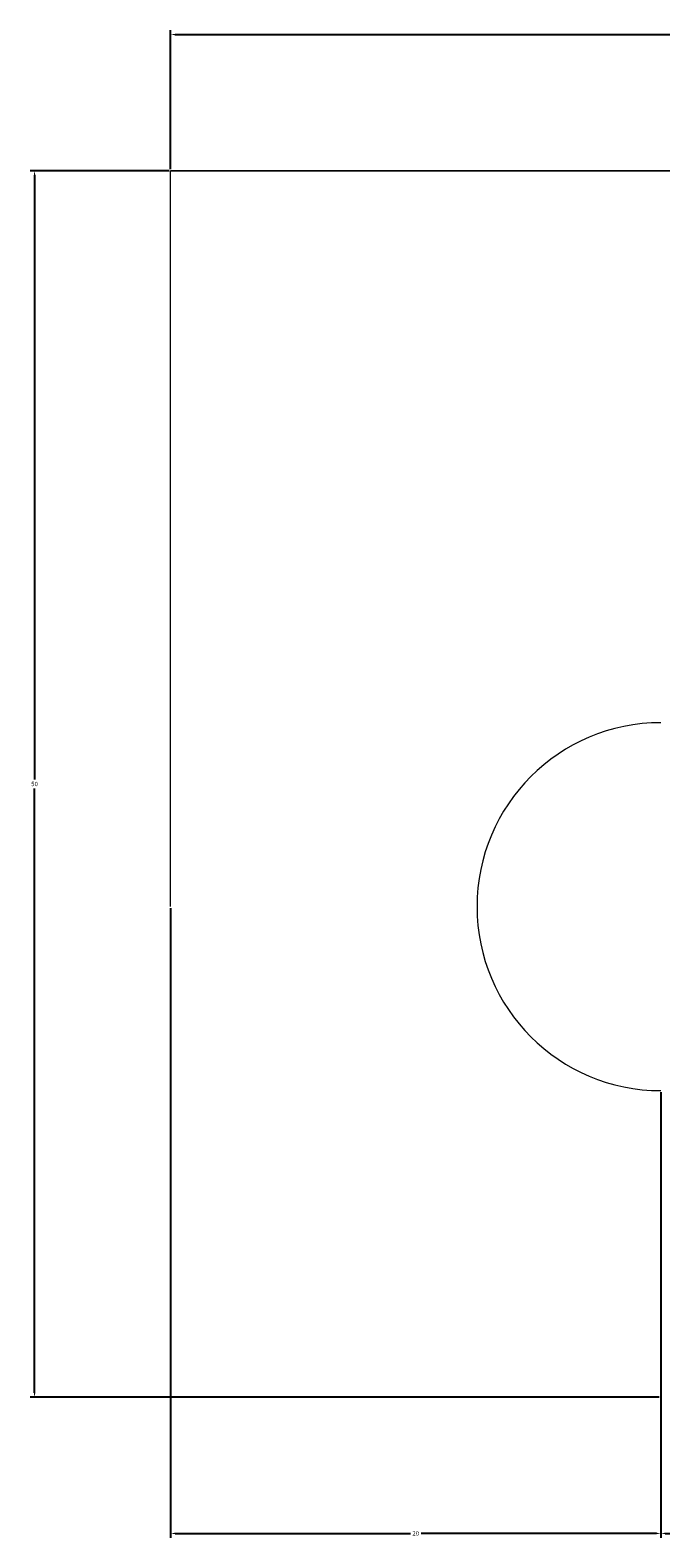
# Model space of a CAD drawing. Units: millimetres. Extents: x 88 to 204, y -56 to 6.
# Tile 1 of 3: x 88 to 114, y -56 to 6. Entities that reach past the tile are written whole.
import ezdxf

# ---------------------------------------------------------------- set-up
doc = ezdxf.new("R2010")
doc.units = ezdxf.units.MM
doc.layers.add('M-CONS', color=8, linetype='Continuous', lineweight=13)
doc.layers.add('M-DIMS', color=2, linetype='Continuous', lineweight=18)
doc.styles.get("Standard").update_dxf_attribs({"font": 'arial.ttf'})
doc.dimstyles.get("Standard").update_dxf_attribs({"dimtxt": 0.18, "dimasz": 0.18, "dimexe": 0.18, "dimexo": 0.0625, "dimgap": 0.09, "dimtad": 0, "dimtih": 1, "dimtoh": 1, "dimdec": 4, "dimzin": 0, "dimdsep": 46, "dimtxsty": 'Standard', "dimcen": 0.09, "dimadec": 0, "dimazin": 0, "dimtfac": 1, "dimtdec": 4, "dimtofl": 0, "dimtmove": 0, "dimatfit": 3, "dimfxl": 1, "dimtolj": 1, "dimtzin": 0, "dimarcsym": 0})

# ---------------------------------------------------------------- blocks, each defined once
blk = doc.blocks.new('*D1')
at = {"layer": 'Defpoints', "color": 0, "transparency": 16777216}
for p in [(198.717, 5.55), (93.717, 0), (198.717, 0)]:
    blk.add_point(p, dxfattribs=at)
at = {"layer": 'M-DIMS', "color": 0, "lineweight": -2, "transparency": 16777216}
for p, q in [((93.717, 0.062), (93.717, 5.73)), ((93.897, 5.55), (145.936, 5.55)), ((198.537, 5.55), (146.498, 5.55)), ((198.717, 0.062), (198.717, 5.73))]:
    blk.add_line(p, q, dxfattribs=at)
at = {"layer": 'M-DIMS', "color": 0, "transparency": 16777216}
for points in [[(93.897, 5.58), (93.897, 5.52), (93.717, 5.55)], [(198.537, 5.58), (198.537, 5.52), (198.717, 5.55)]]:
    blk.add_solid(points, dxfattribs=at)
at = {"layer": 'M-DIMS', "color": 0, "transparency": 16777216, "insert": (146.217, 5.55), "char_height": 0.18, "attachment_point": 5}
blk.add_mtext('\\A1;105', dxfattribs=at)
blk = doc.blocks.new('*D2')
at = {"layer": 'Defpoints', "color": 0, "transparency": 16777216}
for p in [(93.717, 0), (88.167, -50), (113.717, -50)]:
    blk.add_point(p, dxfattribs=at)
at = {"layer": 'M-DIMS', "color": 0, "lineweight": -2, "transparency": 16777216}
for p, q in [((93.654, 0), (87.987, 0)), ((88.167, -0.18), (88.167, -24.818)), ((88.167, -49.82), (88.167, -25.182)), ((113.654, -50), (87.987, -50))]:
    blk.add_line(p, q, dxfattribs=at)
at = {"layer": 'M-DIMS', "color": 0, "transparency": 16777216}
for points in [[(88.137, -0.18), (88.197, -0.18), (88.167, 0)], [(88.137, -49.82), (88.197, -49.82), (88.167, -50)]]:
    blk.add_solid(points, dxfattribs=at)
at = {"layer": 'M-DIMS', "color": 0, "transparency": 16777216, "insert": (88.167, -25), "char_height": 0.18, "attachment_point": 5}
blk.add_mtext('\\A1;50', dxfattribs=at)
blk = doc.blocks.new('*D3')
at = {"layer": 'Defpoints', "color": 0, "transparency": 16777216}
for p in [(93.717, -30), (113.717, -50), (113.717, -55.55)]:
    blk.add_point(p, dxfattribs=at)
at = {"layer": 'M-DIMS', "color": 0, "lineweight": -2, "transparency": 16777216}
for p, q in [((93.717, -30.062), (93.717, -55.73)), ((113.717, -50.062), (113.717, -55.73)), ((93.897, -55.55), (103.497, -55.55)), ((113.537, -55.55), (103.937, -55.55))]:
    blk.add_line(p, q, dxfattribs=at)
at = {"layer": 'M-DIMS', "color": 0, "transparency": 16777216}
for points in [[(93.897, -55.52), (93.897, -55.58), (93.717, -55.55)], [(113.537, -55.52), (113.537, -55.58), (113.717, -55.55)]]:
    blk.add_solid(points, dxfattribs=at)
at = {"layer": 'M-DIMS', "color": 0, "transparency": 16777216, "insert": (103.717, -55.55), "char_height": 0.18, "attachment_point": 5}
blk.add_mtext('\\A1;20', dxfattribs=at)
blk = doc.blocks.new('*D4')
at = {"layer": 'Defpoints', "color": 0, "transparency": 16777216}
for p in [(113.717, -37.5), (143.717, -37.5), (143.717, -55.55)]:
    blk.add_point(p, dxfattribs=at)
at = {"layer": 'M-DIMS', "color": 0, "lineweight": -2, "transparency": 16777216}
for p, q in [((113.717, -37.562), (113.717, -55.73)), ((143.717, -37.562), (143.717, -55.73)), ((113.897, -55.55), (128.498, -55.55)), ((143.537, -55.55), (128.935, -55.55))]:
    blk.add_line(p, q, dxfattribs=at)
at = {"layer": 'M-DIMS', "color": 0, "transparency": 16777216}
for points in [[(113.897, -55.52), (113.897, -55.58), (113.717, -55.55)], [(143.537, -55.52), (143.537, -55.58), (143.717, -55.55)]]:
    blk.add_solid(points, dxfattribs=at)
at = {"layer": 'M-DIMS', "color": 0, "transparency": 16777216, "insert": (128.717, -55.55), "char_height": 0.18, "attachment_point": 5}
blk.add_mtext('\\A1;30', dxfattribs=at)

msp = doc.modelspace()

# ---------------------------------------------------------------- linework, layer by layer
at = {"layer": 'M-CONS', "extrusion": (0, -1, 0)}
for p, q in [((163.717, 0, 52.588), (93.717, 0, 52.588)), ((93.717, 0, 72.588), (163.717, 0, 72.588)), ((93.717, 0, 72.588), (93.717, 0, 112.588))]:
    msp.add_line(p, q, dxfattribs=at)
at = {"layer": 'M-CONS'}
for p, q in [((93.717, 0, 52.588), (93.717, 0, 62.588)), ((93.717, 0, 62.588), (163.717, 0, 62.588)), ((93.717, -30, 62.588), (93.717, 0, 62.588))]:
    msp.add_line(p, q, dxfattribs=at)
msp.add_arc((113.717, -30, 62.588), 7.5, 90, 270, dxfattribs=at)

# ---------------------------------------------------------------- dimensions: what is measured, and where the dimension line sits
at = {"layer": 'M-DIMS'}
for base, p1, p2, picture, middle in [((198.717, 5.55), (93.717, 0), (198.717, 0), '*D1', (146.217, 5.55)), ((113.717, -55.55), (93.717, -30), (113.717, -50), '*D3', (103.717, -55.55)), ((143.717, -55.55), (113.717, -37.5), (143.717, -37.5), '*D4', (128.717, -55.55))]:
    dim = msp.add_linear_dim(base=base, p1=p1, p2=p2, dimstyle='Standard', override={"dimdec": 0, "dimlfac": 1, "dimrnd": 0, "dimzin": 0, "dimdsep": 46, "dimlunit": 2}, dxfattribs=at)
    dim.commit()
    dim.dimension.update_dxf_attribs({"geometry": picture, "text_midpoint": middle})
dim = msp.add_linear_dim(base=(88.167, -50), p1=(93.717, 0), p2=(113.717, -50), angle=90, dimstyle='Standard', override={"dimdec": 0, "dimlfac": 1, "dimrnd": 0, "dimzin": 0, "dimdsep": 46, "dimlunit": 2}, dxfattribs=at)
dim.commit()
dim.dimension.update_dxf_attribs({"geometry": '*D2', "text_midpoint": (88.167, -25)})

doc.saveas('drawing.dxf')
